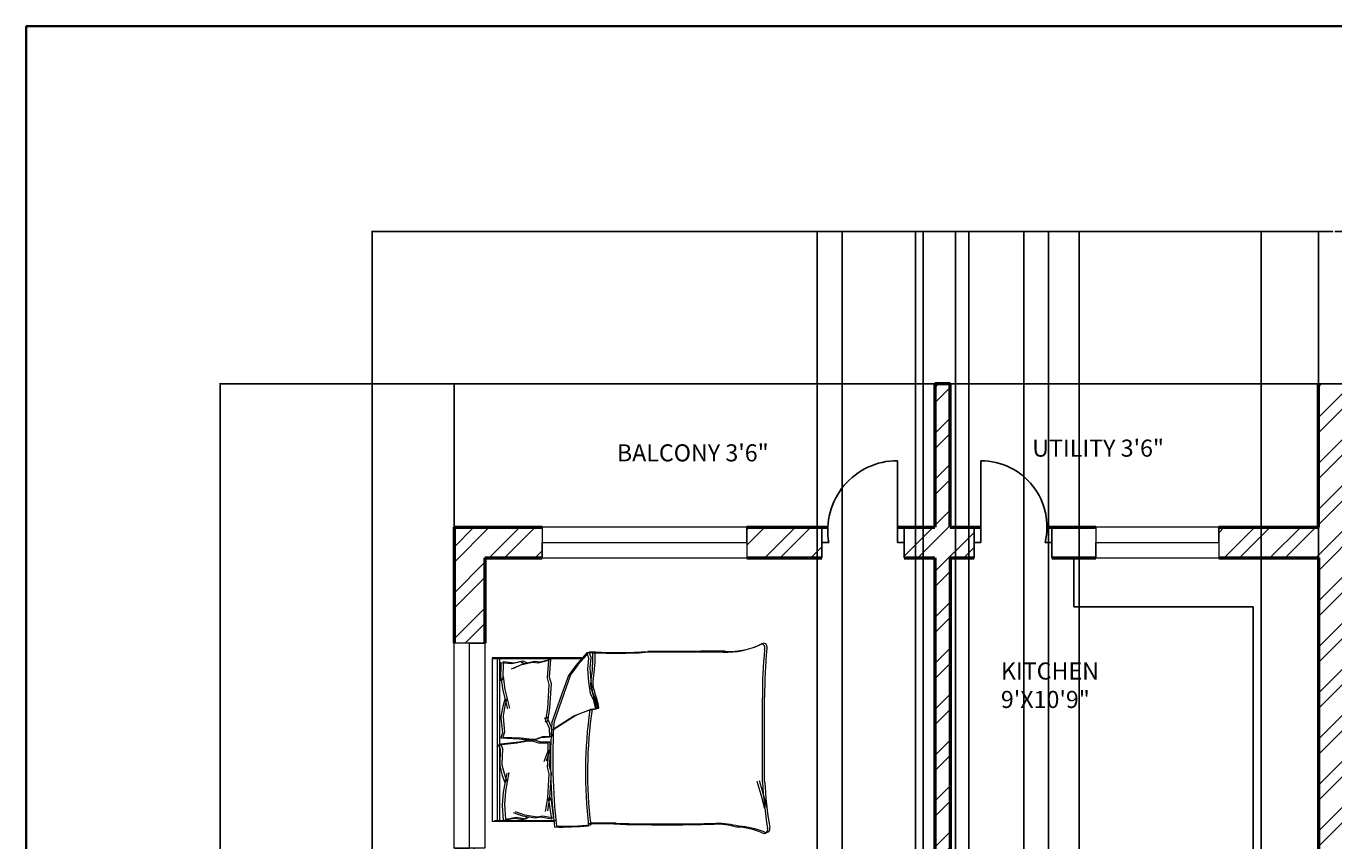
# Model space of a CAD drawing. Units: inches. Extents: x 1980 to 2738, y 1471 to 2568.
# Tile 19 of 22: x 1980 to 2363, y 2329 to 2568. Entities that reach past the tile are written whole.
import ezdxf

# ---------------------------------------------------------------- set-up
doc = ezdxf.new("R2010")
doc.units = ezdxf.units.IN
for name, color, linetype, lineweight in [('A-ANNO-DIMS', 2, 'Continuous', 18), ('A-ANNO-TTLB', 7, 'Continuous', 35), ('A-AREA-IDEN', 7, 'Continuous', 18), ('A-DOOR', 31, 'Continuous', 25), ('A-FLOR-BALC', 7, 'Continuous', 25), ('A-FLOR-CASE', 8, 'Continuous', 25), ('A-FURN', 8, 'Continuous', 18), ('A-GLAZ', 141, 'Continuous', 18), ('A-WALL', 7, 'Continuous', 50)]:
    doc.layers.add(name, color=color, linetype=linetype, lineweight=lineweight)
doc.layers.add('A-WALL-PATT', color=9, linetype='Continuous', lineweight=13, true_color=0xd19cc7)
doc.styles.get("Standard").update_dxf_attribs({"font": 'arial.ttf'})
doc.dimstyles.get("Standard").update_dxf_attribs({"dimtxt": 0.18, "dimasz": 0.18, "dimexe": 0.18, "dimexo": 0.0625, "dimgap": 0.09, "dimtad": 0, "dimtih": 1, "dimtoh": 1, "dimdec": 4, "dimzin": 0, "dimdsep": 46, "dimtxsty": 'Standard', "dimcen": 0.09, "dimadec": 0, "dimazin": 0, "dimtfac": 1, "dimtdec": 4, "dimtofl": 0, "dimtmove": 0, "dimatfit": 3, "dimfxl": 1, "dimtolj": 1, "dimtzin": 0, "dimarcsym": 0})

# ---------------------------------------------------------------- blocks, each defined once
blk = doc.blocks.new('BED-DOUBLE')
for p, q in [((0, 51.49), (0.64, 51.49)), ((0, 51.27), (26.61, 51.27)), ((0, 51.27), (26.61, 51.27)), ((0, 51.27), (0, 3.48)), ((0.64, 51.49), (27.25, 51.49)), ((0.64, 51.49), (27.25, 51.49)), ((1.53, 3.48), (1.53, 51.27)), ((1.53, 3.48), (1.53, 51.27)), ((2.17, 3.7), (2.17, 51.49)), ((2.17, 3.7), (2.17, 51.49)), ((2.56, 50.11), (2.46, 44.71)), ((2.56, 50.11), (2.46, 44.71)), ((2.56, 50.11), (5.77, 49.73)), ((2.56, 50.11), (5.77, 49.73)), ((3.2, 50.34), (3.1, 44.94)), ((3.2, 50.34), (3.1, 44.94)), ((3.2, 50.34), (6.41, 49.96)), ((3.2, 50.34), (6.41, 49.96)), ((5.77, 49.73), (8.34, 50.33)), ((5.77, 49.73), (8.34, 50.33)), ((6.41, 49.96), (8.98, 50.56)), ((6.41, 49.96), (8.98, 50.56)), ((11.83, 50.11), (8.26, 49.31)), ((11.83, 50.11), (8.26, 49.31)), ((8.34, 50.33), (9.38, 49.81)), ((8.34, 50.33), (9.38, 49.81)), ((12.47, 50.34), (8.9, 49.54)), ((12.47, 50.34), (8.9, 49.54)), ((8.98, 50.56), (10.02, 50.04)), ((8.98, 50.56), (10.02, 50.04)), ((13.43, 49.92), (11.83, 50.11)), ((13.43, 49.92), (11.83, 50.11)), ((14.07, 50.15), (12.47, 50.34)), ((14.07, 50.15), (12.47, 50.34)), ((16.57, 50.7), (13.43, 49.92)), ((16.57, 50.7), (13.43, 49.92)), ((17.21, 50.93), (14.07, 50.15)), ((17.21, 50.93), (14.07, 50.15)), ((16.17, 45.57), (16.57, 50.7)), ((16.17, 45.57), (16.57, 50.7)), ((16.81, 45.8), (17.21, 50.93)), ((16.81, 45.79), (17.21, 50.93)), ((27.75, 52.87), (24.5, 49.16)), ((27.75, 52.87), (24.5, 49.16)), ((28.38, 53.1), (25.13, 49.39)), ((28.38, 53.1), (25.13, 49.39)), ((29.49, 52.95), (27.75, 52.87, 3.87)), ((29.49, 52.95), (27.75, 52.87, 3.87)), ((28.36, 51.33), (27.75, 52.87)), ((28.36, 51.33), (27.75, 52.87)), ((28.06, 48.23), (28.36, 51.33)), ((28.06, 48.23), (28.36, 51.33)), ((30.13, 53.18), (28.38, 53.1, 3.87)), ((30.13, 53.18), (28.38, 53.1, 3.87)), ((29, 51.56), (28.38, 53.1)), ((29, 51.56), (28.38, 53.1)), ((28.69, 48.46), (29, 51.56)), ((28.69, 48.46), (29, 51.56)), ((8.26, 49.31), (5.58, 48.13)), ((8.26, 49.31), (5.58, 48.13)), ((8.9, 49.54), (6.22, 48.36)), ((8.9, 49.54), (6.22, 48.36)), ((22.33, 46.22), (20.32, 40.64)), ((22.33, 46.22), (20.32, 40.64)), ((22.97, 46.45), (20.96, 40.87)), ((22.97, 46.45), (20.96, 40.87)), ((24.5, 49.16), (22.33, 46.22)), ((24.5, 49.16), (22.33, 46.22)), ((25.13, 49.39), (22.97, 46.45)), ((25.13, 49.39), (22.97, 46.45)), ((28.36, 44.36), (28.06, 48.23)), ((28.36, 44.36), (28.06, 48.23)), ((29, 44.59), (28.69, 48.46)), ((29, 44.59), (28.69, 48.46)), ((2.46, 44.71), (2.54, 45.71)), ((2.46, 44.71), (2.54, 45.71)), ((2.54, 45.71), (3.07, 41.91)), ((2.54, 45.71), (3.07, 41.91)), ((3.1, 44.94), (3.18, 45.94)), ((3.1, 44.94), (3.18, 45.94)), ((3.18, 45.94), (3.71, 42.14)), ((3.18, 45.94), (3.71, 42.14)), ((16.73, 43.61), (16.17, 45.57)), ((16.73, 43.61), (16.17, 45.57)), ((16.29, 36.6), (16.73, 43.61)), ((16.29, 36.6), (16.73, 43.61)), ((17.37, 43.83), (16.81, 45.8)), ((17.37, 43.83), (16.81, 45.79)), ((16.93, 36.82), (17.37, 43.83)), ((16.93, 36.82), (17.37, 43.83)), ((28.83, 40.95), (28.36, 44.36)), ((28.83, 40.95), (28.36, 44.36)), ((29.47, 41.18), (29, 44.59)), ((29.47, 41.18), (29, 44.59)), ((3.07, 41.91), (4.42, 36.5)), ((3.07, 41.91), (4.42, 36.5)), ((3.67, 39.2), (3.08, 37.14)), ((3.67, 39.2), (3.08, 37.14)), ((3.71, 42.14), (5.06, 36.72)), ((3.71, 42.14), (5.06, 36.72)), ((4.31, 39.43), (3.72, 37.36)), ((4.31, 39.43), (3.72, 37.36)), ((20.32, 40.64), (17.38, 32.31)), ((20.32, 40.64), (17.38, 32.31)), ((20.96, 40.87), (18.02, 32.53)), ((20.96, 40.87), (18.02, 32.53)), ((29.76, 38.94), (28.83, 40.95)), ((29.76, 38.94), (28.83, 40.95)), ((30.4, 39.17), (29.47, 41.18)), ((30.4, 39.17), (29.47, 41.18)), ((30.38, 36.46), (29.76, 38.94)), ((30.38, 36.46), (29.76, 38.94)), ((31.02, 36.69), (30.4, 39.17)), ((31.02, 36.69), (30.4, 39.17)), ((79.24, 15.06), (79.24, 39.68)), ((79.24, 15.06), (79.24, 39.68)), ((79.88, 15.29), (79.88, 39.91)), ((79.88, 15.29), (79.88, 39.91)), ((3.08, 37.14), (2.54, 34.2)), ((3.08, 37.14), (2.54, 34.2)), ((3.72, 37.36), (3.18, 34.43)), ((3.72, 37.36), (3.18, 34.43)), ((15.63, 32.56), (16.29, 36.6)), ((15.63, 32.56), (16.29, 36.6)), ((16.27, 32.79), (16.93, 36.82)), ((16.27, 32.79), (16.93, 36.82)), ((18.02, 30.49), (24.52, 34.68)), ((18.02, 30.49), (24.52, 34.68)), ((23.88, 34.45), (28.36, 36.15)), ((23.88, 34.45), (28.36, 36.15)), ((24.52, 34.68), (29, 36.38)), ((24.52, 34.68), (29, 36.38)), ((28.36, 36.15), (30.38, 36.46)), ((28.36, 36.15), (30.38, 36.46)), ((29, 36.38), (31.02, 36.69)), ((29, 36.38), (31.02, 36.69)), ((2.54, 34.2), (2.56, 33.88)), ((2.54, 34.2), (2.56, 33.88)), ((2.56, 33.88), (2.98, 29.46)), ((2.56, 33.88), (2.98, 29.46)), ((3.18, 34.43), (3.2, 34.11)), ((3.18, 34.43), (3.2, 34.11)), ((3.2, 34.11), (3.62, 29.68)), ((3.2, 34.11), (3.62, 29.68)), ((16.74, 30.75), (15.45, 33.82)), ((16.74, 30.75), (15.45, 33.82)), ((17.38, 30.98), (16.09, 34.05)), ((17.38, 30.98), (16.09, 34.05)), ((16.89, 28.3), (16.74, 30.75)), ((16.89, 28.3), (16.74, 30.75)), ((17.38, 30.26), (23.88, 34.45)), ((17.38, 30.26), (23.88, 34.45)), ((17.53, 28.53), (17.38, 30.98)), ((17.53, 28.53), (17.38, 30.98)), ((2.98, 29.46), (2.49, 27.98)), ((2.98, 29.46), (2.49, 27.98)), ((2.49, 27.98), (7.87, 27.73)), ((2.49, 27.98), (7.87, 27.73)), ((3.62, 29.68), (3.13, 28.21)), ((3.62, 29.68), (3.13, 28.21)), ((3.13, 28.21), (8.51, 27.96)), ((3.13, 28.21), (8.51, 27.96)), ((7.22, 26.56), (10.4, 27.14)), ((7.22, 26.56), (10.4, 27.14)), ((7.86, 26.79), (11.04, 27.37)), ((7.86, 26.79), (11.04, 27.37)), ((7.87, 27.73), (11.08, 27.36)), ((7.87, 27.73), (11.08, 27.35)), ((8.51, 27.96), (11.72, 27.58)), ((8.51, 27.96), (11.72, 27.58)), ((10.4, 27.14), (11.7, 27.14)), ((10.4, 27.14), (11.7, 27.14)), ((11.04, 27.37), (12.34, 27.37)), ((11.04, 27.37), (12.34, 27.37)), ((11.08, 27.36), (12.38, 27.44)), ((11.08, 27.35), (12.38, 27.44)), ((11.7, 27.14), (13.58, 26.56)), ((11.7, 27.14), (13.58, 26.56)), ((11.72, 27.58), (13.02, 27.66)), ((11.72, 27.58), (13.02, 27.66)), ((12.34, 27.37), (14.22, 26.79)), ((12.34, 27.37), (14.22, 26.79)), ((12.38, 27.44), (14.22, 28.13)), ((12.38, 27.44), (14.22, 28.13)), ((13.02, 27.66), (14.86, 28.36)), ((13.02, 27.66), (14.86, 28.36)), ((14.22, 28.13), (16.89, 28.3)), ((14.22, 28.13), (16.89, 28.3)), ((14.86, 28.36), (17.53, 28.53)), ((14.86, 28.36), (17.53, 28.53)), ((1.87, 25.98), (7.22, 26.56)), ((1.87, 25.98), (7.22, 26.56)), ((2.45, 24.54), (1.87, 25.98)), ((2.45, 24.54), (1.87, 25.98)), ((2.3, 20.09), (2.45, 24.54)), ((2.3, 20.09), (2.45, 24.54)), ((2.51, 26.21), (7.86, 26.79)), ((2.51, 26.21), (7.86, 26.79)), ((3.09, 24.77), (2.51, 26.21)), ((3.09, 24.77), (2.51, 26.21)), ((2.94, 20.32), (3.09, 24.77)), ((2.94, 20.32), (3.09, 24.77)), ((13.58, 26.56), (16.26, 26.56)), ((13.58, 26.56), (16.26, 26.56)), ((14.22, 26.79), (16.9, 26.79)), ((14.22, 26.79), (16.9, 26.79)), ((16.26, 24.1), (15.17, 20.96)), ((16.26, 24.1), (15.17, 20.96)), ((16.9, 24.33), (15.81, 21.19)), ((16.9, 24.33), (15.81, 21.19)), ((16.17, 19.38), (16.57, 24.52)), ((16.17, 19.38), (16.57, 24.52)), ((16.26, 26.56), (16.26, 24.1)), ((16.26, 26.56), (16.26, 24.1)), ((16.81, 19.61), (17.21, 24.74)), ((16.81, 19.61), (17.21, 24.74)), ((16.9, 26.79), (16.9, 24.33)), ((16.9, 26.79), (16.9, 24.33)), ((2.3, 19.77), (2.3, 20.09)), ((2.3, 19.77), (2.3, 20.09)), ((3.03, 16.88), (2.3, 19.77)), ((3.03, 16.88), (2.3, 19.77)), ((2.94, 20), (2.94, 20.32)), ((2.94, 20), (2.94, 20.32)), ((3.67, 17.11), (2.94, 20)), ((3.67, 17.11), (2.94, 20)), ((16.73, 17.42), (16.17, 19.38)), ((16.73, 17.42), (16.17, 19.38)), ((17.37, 17.65), (16.81, 19.61)), ((17.37, 17.65), (16.81, 19.61)), ((3.75, 14.86), (3.03, 16.88)), ((3.75, 14.85), (3.03, 16.88)), ((3.32, 12.11), (4.33, 17.6)), ((3.32, 12.11), (4.33, 17.6)), ((4.39, 15.08), (3.67, 17.11)), ((4.39, 15.08), (3.67, 17.11)), ((3.96, 12.34), (4.97, 17.83)), ((3.96, 12.34), (4.97, 17.83)), ((16.29, 10.41), (16.73, 17.42)), ((16.29, 10.41), (16.73, 17.42)), ((16.93, 10.64), (17.37, 17.65)), ((16.93, 10.64), (17.37, 17.65)), ((3.03, 8.29), (3.32, 12.11)), ((3.03, 8.28), (3.32, 12.11)), ((3.67, 8.51), (3.96, 12.34)), ((3.67, 8.51), (3.96, 12.34)), ((3.01, 8.18), (3.03, 8.29)), ((3.01, 8.18), (3.03, 8.28)), ((3.34, 3.9), (3.01, 8.18)), ((3.34, 3.9), (3.01, 8.18)), ((3.65, 8.41), (3.67, 8.51)), ((3.65, 8.41), (3.67, 8.51)), ((3.98, 4.13), (3.65, 8.41)), ((3.98, 4.13), (3.65, 8.41)), ((15.63, 6.38), (16.29, 10.41)), ((15.63, 6.38), (16.29, 10.41)), ((16.27, 6.61), (16.93, 10.64)), ((16.27, 6.61), (16.93, 10.64)), ((16.29, 10.41), (16.62, 9.28)), ((16.29, 10.41), (16.62, 9.28)), ((16.62, 9.28), (17.34, 4.18)), ((16.62, 9.28), (17.34, 4.18)), ((16.93, 10.64), (17.26, 9.51)), ((16.93, 10.64), (17.26, 9.51)), ((17.26, 9.51), (17.98, 4.41)), ((17.26, 9.51), (17.98, 4.41)), ((3.32, 3.89), (6.5, 4.47)), ((3.32, 3.89), (6.5, 4.47)), ((3.96, 4.12), (7.14, 4.7)), ((3.96, 4.12), (7.14, 4.7)), ((8.95, 5.05), (6.21, 6.06)), ((8.95, 5.05), (6.21, 6.06)), ((6.5, 4.47), (9.1, 4.04)), ((6.5, 4.47), (9.1, 4.04)), ((9.59, 5.28), (6.85, 6.29)), ((9.59, 5.28), (6.85, 6.29)), ((7.14, 4.7), (9.74, 4.27)), ((7.14, 4.7), (9.74, 4.27)), ((12.57, 4.47), (8.95, 5.05)), ((12.57, 4.47), (8.95, 5.05)), ((9.1, 4.04), (10.11, 4.62)), ((9.1, 4.04), (10.11, 4.62)), ((13.21, 4.7), (9.59, 5.28)), ((13.21, 4.7), (9.59, 5.28)), ((9.74, 4.27), (10.75, 4.85)), ((9.74, 4.27), (10.75, 4.85)), ((14.16, 4.76), (12.57, 4.47)), ((14.16, 4.76), (12.57, 4.47)), ((14.8, 4.99), (13.21, 4.7)), ((14.8, 4.99), (13.21, 4.7)), ((17.34, 4.18), (14.16, 4.76)), ((17.34, 4.18), (14.16, 4.76)), ((17.98, 4.41), (14.8, 4.99)), ((17.98, 4.41), (14.8, 4.99)), ((18.11, 3.48), (0, 3.48)), ((18.11, 3.48), (0, 3.48)), ((18.75, 3.7), (0.64, 3.7)), ((18.75, 3.7), (0.64, 3.7))]:
    blk.add_line(p, q)
for centre, radius, start, end in [((68.67, 76.16), 23.07, 267.4714, 296.4681), ((68.67, 76.16), 23.07, 267.4714, 296.4681), ((69.31, 76.39), 23.07, 267.4714, 296.4681), ((69.31, 76.39), 23.07, 267.4714, 296.4681), ((78.87, 54.41), 1.1, 332.6588, 86.02), ((78.87, 54.41), 1.1, 332.6588, 86.02), ((212.28, 41.15), 133.04, 174.4998, 180.6351), ((212.28, 41.15), 133.04, 174.4998, 180.6351), ((79.51, 54.64), 1.1, 332.6588, 86.02), ((79.51, 54.64), 1.1, 332.6588, 86.02), ((212.92, 41.38), 133.04, 174.4998, 180.6351), ((212.92, 41.38), 133.04, 174.4998, 180.6351), ((-6.66, 51.33), 36.18, 349.8763, 2.5657), ((-6.66, 51.33), 36.18, 349.8763, 2.5657), ((36.31, 182.27), 129.5, 266.9791, 273.8365), ((36.31, 182.27), 129.5, 266.9791, 273.8365), ((-6.02, 51.56), 36.18, 349.8763, 2.5657), ((-6.02, 51.56), 36.18, 349.8763, 2.5657), ((36.95, 182.49), 129.5, 266.9791, 273.8365), ((36.95, 182.49), 129.5, 266.9791, 273.8365), ((67.82, -4508.74), 4561.86, 90.00217, 90.28689), ((67.82, -4508.74), 4561.86, 90.00217, 90.28689), ((68.46, -4508.51), 4561.86, 90.00217, 90.28689), ((68.46, -4508.52), 4561.86, 90.00217, 90.28689), ((35.07, 43.74), 6.22, 168.6608, 203.7384), ((35.07, 43.74), 6.22, 168.6608, 203.7384), ((35.71, 43.97), 6.22, 168.6608, 203.7384), ((35.71, 43.97), 6.22, 168.6608, 203.7384), ((1.48, 31.15), 29.65, 10.6617, 19.8806), ((1.48, 31.15), 29.65, 10.6617, 19.8806), ((2.12, 31.38), 29.65, 10.6617, 19.8806), ((2.12, 31.38), 29.65, 10.6617, 19.8806), ((156.32, 17.76), 129.02, 171.7845, 186.9006), ((156.32, 17.76), 129.02, 171.7845, 186.9006), ((156.96, 17.98), 129.02, 171.7845, 186.9006), ((156.96, 17.98), 129.02, 171.7845, 186.9006), ((30.44, 36.64), 0.185, 250.2464, 1.1377), ((30.44, 36.64), 0.185, 250.2464, 1.1377), ((31.08, 36.86), 0.185, 250.2464, 1.1377), ((31.08, 36.86), 0.185, 250.2464, 1.1377), ((182.05, 21.36), 164.97, 176.0865, 186.7821), ((182.05, 21.36), 164.97, 176.0865, 186.7821), ((182.69, 21.59), 164.97, 176.0865, 186.7821), ((182.69, 21.59), 164.97, 176.0865, 186.7821), ((-23.07, -16.99), 106.46, 13.3832, 17.7053), ((-23.07, -16.99), 106.46, 13.3832, 17.7053), ((-23.71, -17.22), 106.46, 13.3832, 17.7053), ((-23.71, -17.22), 106.46, 13.3832, 17.7053), ((200.84, 21.43), 121.76, 182.9958, 189.4091), ((200.84, 21.43), 121.76, 182.9958, 189.4091), ((201.48, 21.66), 121.76, 182.9958, 189.4091), ((201.48, 21.66), 121.76, 182.9958, 189.4091), ((20.1, 85.16), 83.31, 268.7218, 275.604), ((20.1, 85.16), 83.31, 268.7218, 275.604), ((20.74, 85.39), 83.31, 268.7218, 275.604), ((20.74, 85.39), 83.31, 268.7218, 275.604), ((31.17, -167.31), 170.11, 88.4762, 91.0082), ((31.17, -167.31), 170.11, 88.4762, 91.0082), ((31.81, -167.08), 170.11, 88.4762, 91.0082), ((31.81, -167.08), 170.11, 88.4762, 91.0082), ((50.61, 484.82), 482.31, 268.2277, 271.7185), ((50.61, 484.82), 482.31, 268.2277, 271.7185), ((51.25, 485.05), 482.31, 268.2277, 271.7185), ((51.25, 485.05), 482.31, 268.2277, 271.7185), ((64.51, -26.9), 29.63, 76.0648, 88.9113), ((64.51, -26.9), 29.63, 76.0648, 88.9113), ((65.15, -26.67), 29.63, 76.0648, 88.9113), ((65.15, -26.67), 29.63, 76.0648, 88.9113), ((70.28, -21.66), 23.56, 67.9751, 86.652), ((70.28, -21.66), 23.56, 67.9751, 86.652), ((70.91, -21.43), 23.56, 67.9751, 86.652), ((70.91, -21.43), 23.56, 67.9751, 86.652), ((79.72, 1.09), 1.09, 236.1736, 23.4781), ((79.72, 1.09), 1.09, 236.1736, 23.4781), ((80.36, 1.32), 1.09, 236.1736, 23.4781), ((80.36, 1.32), 1.09, 236.1736, 23.4781)]:
    blk.add_arc(centre, radius, start, end)
blk = doc.blocks.new('WIN-60IN-WALL')
for p, q in [((0, 9), (0, 0)), ((60, 9), (0, 9)), ((60, 4.5), (60, 9)), ((60, 9), (60, 0)), ((0, 0), (0, 4.5)), ((0, 4.5), (60, 4.5)), ((0, 0), (60, 0))]:
    blk.add_line(p, q)
blk = doc.blocks.new('*D35')
at = {"layer": 'A-ANNO-DIMS', "color": 0, "lineweight": -2, "transparency": 16777216}
for p, q in [((2081.08, 2291.77), (2081.08, 2507.54)), ((2081.26, 2507.36), (2362.79, 2507.36)), ((2644.9, 2507.36), (2363.37, 2507.36)), ((2645.08, 2291.77), (2645.08, 2507.54))]:
    blk.add_line(p, q, dxfattribs=at)
at = {"layer": 'A-ANNO-DIMS', "color": 0, "transparency": 16777216}
for points in [[(2081.26, 2507.39), (2081.26, 2507.33), (2081.08, 2507.36)], [(2644.9, 2507.39), (2644.9, 2507.33), (2645.08, 2507.36)]]:
    blk.add_solid(points, dxfattribs=at)
at = {"layer": 'Defpoints', "color": 0, "transparency": 16777216}
for p in [(2645.08, 2507.36), (2081.08, 2291.71), (2645.08, 2291.71)]:
    blk.add_point(p, dxfattribs=at)
at = {"layer": 'A-ANNO-DIMS', "color": 0, "transparency": 16777216, "insert": (2363.08, 2507.36), "char_height": 0.18, "attachment_point": 5}
blk.add_mtext('\\A1;564', dxfattribs=at)
blk = doc.blocks.new('*D36')
at = {"layer": 'A-ANNO-DIMS', "color": 0, "lineweight": -2, "transparency": 16777216}
for p, q in [((2105.02, 2462.71), (2036.25, 2462.71)), ((2036.43, 2462.53), (2036.43, 2053.39)), ((2036.43, 1643.89), (2036.43, 2053.02)), ((2105.02, 1643.71), (2036.25, 1643.71))]:
    blk.add_line(p, q, dxfattribs=at)
at = {"layer": 'A-ANNO-DIMS', "color": 0, "transparency": 16777216}
for points in [[(2036.4, 2462.53), (2036.46, 2462.53), (2036.43, 2462.71)], [(2036.4, 1643.89), (2036.46, 1643.89), (2036.43, 1643.71)]]:
    blk.add_solid(points, dxfattribs=at)
at = {"layer": 'Defpoints', "color": 0, "transparency": 16777216}
for p in [(2036.43, 2462.71), (2105.08, 2462.71), (2105.08, 1643.71)]:
    blk.add_point(p, dxfattribs=at)
at = {"layer": 'A-ANNO-DIMS', "color": 0, "transparency": 16777216, "insert": (2036.43, 2053.21), "char_height": 0.18, "attachment_point": 5}
blk.add_mtext('\\A1;819', dxfattribs=at)
blk = doc.blocks.new('*D44')
at = {"layer": 'A-ANNO-DIMS', "color": 0, "lineweight": -2, "transparency": 16777216}
for p, q in [((2218.88, 1694.77), (2218.88, 2507.54)), ((2219.06, 2507.36), (2229.18, 2507.36)), ((2240.22, 2507.36), (2230.11, 2507.36)), ((2240.4, 1694.77), (2240.4, 2507.54))]:
    blk.add_line(p, q, dxfattribs=at)
at = {"layer": 'A-ANNO-DIMS', "color": 0, "transparency": 16777216}
for points in [[(2219.06, 2507.39), (2219.06, 2507.33), (2218.88, 2507.36)], [(2240.22, 2507.39), (2240.22, 2507.33), (2240.4, 2507.36)]]:
    blk.add_solid(points, dxfattribs=at)
at = {"layer": 'Defpoints', "color": 0, "transparency": 16777216}
for p in [(2240.4, 2507.36), (2218.88, 1694.71), (2240.4, 1694.71)]:
    blk.add_point(p, dxfattribs=at)
at = {"layer": 'A-ANNO-DIMS', "color": 0, "transparency": 16777216, "insert": (2229.64, 2507.36), "char_height": 0.18, "attachment_point": 5}
blk.add_mtext('\\A1;21.525', dxfattribs=at)
blk = doc.blocks.new('*D45')
at = {"layer": 'A-ANNO-DIMS', "color": 0, "lineweight": -2, "transparency": 16777216}
for p, q in [((2255.99, 1694.77), (2255.99, 2507.54)), ((2256.17, 2507.36), (2267.22, 2507.36)), ((2279.21, 2507.36), (2268.15, 2507.36)), ((2279.39, 1694.77), (2279.39, 2507.54))]:
    blk.add_line(p, q, dxfattribs=at)
at = {"layer": 'A-ANNO-DIMS', "color": 0, "transparency": 16777216}
for points in [[(2256.17, 2507.39), (2256.17, 2507.33), (2255.99, 2507.36)], [(2279.21, 2507.39), (2279.21, 2507.33), (2279.39, 2507.36)]]:
    blk.add_solid(points, dxfattribs=at)
at = {"layer": 'Defpoints', "color": 0, "transparency": 16777216}
for p in [(2279.39, 2507.36), (2255.99, 1694.71), (2279.39, 1694.71)]:
    blk.add_point(p, dxfattribs=at)
at = {"layer": 'A-ANNO-DIMS', "color": 0, "transparency": 16777216, "insert": (2267.69, 2507.36), "char_height": 0.18, "attachment_point": 5}
blk.add_mtext('\\A1;23.407', dxfattribs=at)
blk = doc.blocks.new('*D46')
at = {"layer": 'A-ANNO-DIMS', "color": 0, "lineweight": -2, "transparency": 16777216}
for p, q in [((2211.52, 1814.77), (2211.52, 2507.54)), ((2211.7, 2507.36), (2226.69, 2507.36)), ((2242.46, 2507.36), (2227.48, 2507.36)), ((2242.64, 1814.77), (2242.64, 2507.54))]:
    blk.add_line(p, q, dxfattribs=at)
at = {"layer": 'A-ANNO-DIMS', "color": 0, "transparency": 16777216}
for points in [[(2211.7, 2507.39), (2211.7, 2507.33), (2211.52, 2507.36)], [(2242.46, 2507.39), (2242.46, 2507.33), (2242.64, 2507.36)]]:
    blk.add_solid(points, dxfattribs=at)
at = {"layer": 'Defpoints', "color": 0, "transparency": 16777216}
for p in [(2242.64, 2507.36), (2211.52, 1814.71), (2242.64, 1814.71)]:
    blk.add_point(p, dxfattribs=at)
at = {"layer": 'A-ANNO-DIMS', "color": 0, "transparency": 16777216, "insert": (2227.08, 2507.36), "char_height": 0.18, "attachment_point": 5}
blk.add_mtext('\\A1;31.12', dxfattribs=at)
blk = doc.blocks.new('*D50')
at = {"layer": 'A-ANNO-DIMS', "color": 0, "lineweight": -2, "transparency": 16777216}
for p, q in [((2288.43, 1708.09), (2288.43, 2507.54)), ((2288.61, 2507.36), (2314.71, 2507.36)), ((2341.6, 2507.36), (2315.5, 2507.36)), ((2341.78, 1708.09), (2341.78, 2507.54))]:
    blk.add_line(p, q, dxfattribs=at)
at = {"layer": 'A-ANNO-DIMS', "color": 0, "transparency": 16777216}
for points in [[(2288.61, 2507.39), (2288.61, 2507.33), (2288.43, 2507.36)], [(2341.6, 2507.39), (2341.6, 2507.33), (2341.78, 2507.36)]]:
    blk.add_solid(points, dxfattribs=at)
at = {"layer": 'Defpoints', "color": 0, "transparency": 16777216}
for p in [(2341.78, 2507.36), (2288.43, 1708.03), (2341.78, 1708.03)]:
    blk.add_point(p, dxfattribs=at)
at = {"layer": 'A-ANNO-DIMS', "color": 0, "transparency": 16777216, "insert": (2315.11, 2507.36), "char_height": 0.18, "attachment_point": 5}
blk.add_mtext('\\A1;53.34', dxfattribs=at)
blk = doc.blocks.new('*D51')
at = {"layer": 'A-ANNO-DIMS', "color": 0, "lineweight": -2, "transparency": 16777216}
for p, q in [((2341.78, 1708.09), (2341.78, 2507.54)), ((2341.96, 2507.36), (2349.72, 2507.36)), ((2358.4, 2507.36), (2350.63, 2507.36)), ((2358.58, 1694.77), (2358.58, 2507.54))]:
    blk.add_line(p, q, dxfattribs=at)
at = {"layer": 'A-ANNO-DIMS', "color": 0, "transparency": 16777216}
for points in [[(2341.96, 2507.39), (2341.96, 2507.33), (2341.78, 2507.36)], [(2358.4, 2507.39), (2358.4, 2507.33), (2358.58, 2507.36)]]:
    blk.add_solid(points, dxfattribs=at)
at = {"layer": 'Defpoints', "color": 0, "transparency": 16777216}
for p in [(2358.58, 2507.36), (2341.78, 1708.03), (2358.58, 1694.71)]:
    blk.add_point(p, dxfattribs=at)
at = {"layer": 'A-ANNO-DIMS', "color": 0, "transparency": 16777216, "insert": (2350.18, 2507.36), "char_height": 0.18, "attachment_point": 5}
blk.add_mtext('\\A1;16.807', dxfattribs=at)
blk = doc.blocks.new('*D54')
at = {"layer": 'A-ANNO-DIMS', "color": 0, "lineweight": -2, "transparency": 16777216}
for p, q in [((2252.1, 1949.01), (2252.1, 2507.54)), ((2252.28, 2507.36), (2261.78, 2507.36)), ((2272.03, 2507.36), (2262.53, 2507.36)), ((2272.21, 1949.01), (2272.21, 2507.54))]:
    blk.add_line(p, q, dxfattribs=at)
at = {"layer": 'A-ANNO-DIMS', "color": 0, "transparency": 16777216}
for points in [[(2252.28, 2507.39), (2252.28, 2507.33), (2252.1, 2507.36)], [(2272.03, 2507.39), (2272.03, 2507.33), (2272.21, 2507.36)]]:
    blk.add_solid(points, dxfattribs=at)
at = {"layer": 'Defpoints', "color": 0, "transparency": 16777216}
for p in [(2272.21, 2507.36), (2252.1, 1948.95), (2272.21, 1948.95)]:
    blk.add_point(p, dxfattribs=at)
at = {"layer": 'A-ANNO-DIMS', "color": 0, "transparency": 16777216, "insert": (2262.16, 2507.36), "char_height": 0.18, "attachment_point": 5}
blk.add_mtext('\\A1;20.11', dxfattribs=at)

msp = doc.modelspace()

# ---------------------------------------------------------------- hatches: boundary and pattern name
at = {"layer": 'A-WALL-PATT'}
h = msp.add_hatch(dxfattribs=at)
h.set_pattern_fill('ANSI32', color=256)
h.paths.add_polyline_path([(2257.5661, 2416.2064), (2257.5661, 2420.7064), (2250.5833, 2420.7064), (2250.5833, 2462.7064), (2246.0833, 2462.7064), (2246.0833, 2420.7064), (2237.0791, 2420.7064), (2237.0791, 2411.7064), (2246.0833, 2411.7064), (2246.0833, 2291.7064), (2242.6109, 2291.7064), (2242.6109, 2287.2064), (2246.0833, 2287.2064), (2250.5833, 2287.2064), (2250.5833, 2291.7064), (2250.5833, 2411.7064), (2257.5661, 2411.7064)])
h.paths.add_polyline_path([(2387.0396, 2416.2064), (2387.0396, 2420.7064), (2367.5833, 2420.7064), (2367.5833, 2462.7064), (2358.5833, 2462.7064), (2358.5833, 2420.7064), (2329.3087, 2420.7064), (2329.3087, 2411.7064), (2358.5833, 2411.7064), (2358.5833, 2321.7275), (2358.5833, 2309.7064), (2347.3089, 2309.7064), (2293.3089, 2309.7064), (2293.3089, 2259.0771), (2297.8089, 2259.0771), (2297.8089, 2305.2064), (2347.3089, 2305.2064), (2347.3089, 2284.7412), (2351.8089, 2284.7412), (2351.8089, 2305.2064), (2372.3188, 2305.2064), (2372.3761, 2284.3899), (2377.0295, 2284.3899), (2377.0295, 2299.3058), (2377.0295, 2305.2064), (2426.5295, 2305.2064), (2426.5295, 2257.5573), (2431.0295, 2257.5573), (2431.0295, 2309.7064), (2377.0295, 2309.7064), (2367.5833, 2309.7064), (2367.5833, 2321.7275), (2367.5833, 2411.7064), (2387.0396, 2411.7064)])
h.paths.add_polyline_path([(2448.5267, 2416.2064), (2448.5267, 2420.7064), (2423.0396, 2420.7064), (2423.0396, 2411.7064), (2448.5267, 2411.7064)])
h.paths.add_polyline_path([(2130.9128, 2416.2064), (2130.9128, 2420.7064), (2105.0833, 2420.7064), (2105.0833, 2386.6942), (2114.0833, 2386.6942), (2114.0833, 2411.7064), (2130.9128, 2411.7064)])
h.paths.add_polyline_path([(2212.9478, 2420.7064), (2190.9128, 2420.7064), (2190.9128, 2411.7064), (2212.9478, 2411.7064), (2212.9478, 2416.2064)])
h.paths.add_polyline_path([(2114.0833, 2326.6942), (2105.0833, 2326.6942), (2105.0833, 2291.7064), (2081.0833, 2291.7064), (2081.0833, 2287.2064), (2105.0833, 2287.2064), (2105.0833, 2276.1935), (2114.0833, 2276.1935), (2114.0833, 2287.2064), (2166.3825, 2287.2064), (2166.3825, 2289.4564), (2166.3825, 2291.7064), (2114.0833, 2291.7064)])
h.paths.add_polyline_path([(2114.0833, 2252.1935), (2105.0833, 2252.1935), (2105.0833, 2233.2064), (2081.0833, 2233.2064), (2081.0833, 2228.7064), (2105.0833, 2228.7064), (2105.0833, 2213.4478), (2114.0833, 2213.4478), (2114.0833, 2228.7064), (2195.0833, 2228.7064), (2199.5833, 2228.7064), (2208.4455, 2228.7064), (2208.4455, 2230.9564), (2208.4455, 2233.2064), (2199.5833, 2233.2064), (2199.5833, 2287.2064), (2206.8904, 2287.2064), (2206.8904, 2289.4564), (2206.8904, 2291.7064), (2189.446, 2291.7064), (2189.446, 2289.4564), (2189.446, 2287.2064), (2195.0833, 2287.2064), (2195.0833, 2233.2064), (2114.0833, 2233.2064)])
h.paths.add_polyline_path([(2114.0833, 2153.4478), (2109.5833, 2153.4478), (2105.0833, 2153.4478), (2105.0833, 2135.2374), (2114.0833, 2135.2374)], flags=17)
h.paths.add_polyline_path([(2135.9619, 2095.4081), (2140.1805, 2095.4081), (2140.1805, 2104.2064), (2114.0833, 2104.2064), (2114.0833, 2110.3997), (2109.5833, 2110.3997), (2105.0833, 2110.3997), (2105.0833, 2104.2064), (2081.0833, 2104.2064), (2081.0833, 2099.7064), (2105.0833, 2099.7064), (2127.5416, 2099.8532), (2127.5416, 2056.9393), (2136.2133, 2056.9393)], flags=17)
h.paths.add_polyline_path([(2255.4895, 2104.2064), (2250.5833, 2104.2064), (2250.5833, 2233.2064), (2246.0833, 2233.2064), (2242.4941, 2233.2064), (2242.4941, 2228.7064), (2246.0833, 2228.7064), (2246.0833, 2104.2064), (2163.6825, 2104.2064), (2163.6825, 2099.8072), (2163.6825, 2095.4081), (2191.4325, 2095.4081), (2191.4325, 2011.2064), (2186.0833, 2011.2064), (2136.5143, 2010.8824), (2136.3702, 2032.9403), (2131.9559, 2032.9115), (2127.5416, 2032.8826), (2127.5416, 2006.7064), (2105.0833, 2006.7064), (2081.0833, 2006.7064), (2081.0833, 2002.2064), (2105.0833, 2002.2064), (2105.0833, 1995.9329), (2114.0833, 1995.9329), (2114.0833, 2002.2064), (2246.0833, 2002.2064), (2246.0833, 1877.7064), (2242.1358, 1877.7064), (2242.1358, 1873.2064), (2250.5833, 1873.2064), (2250.5833, 2002.2064), (2255.3335, 2002.2064), (2255.3335, 2011.2064), (2195.9325, 2011.2064), (2195.9325, 2095.2064), (2255.4895, 2095.2064), (2255.4895, 2099.5471)])
h.paths.add_polyline_path([(2199.5833, 1873.2064), (2209.827, 1873.2064), (2209.827, 1875.4564), (2209.827, 1877.7064), (2114.0833, 1877.7064), (2114.0833, 1890.0968), (2105.0833, 1890.0968), (2105.0833, 1877.7064), (2081.0833, 1877.7064), (2081.0833, 1873.2064), (2105.0833, 1873.2064), (2105.0833, 1857.7279), (2114.0833, 1857.7279), (2114.0833, 1873.2064), (2195.0833, 1873.2064), (2195.0833, 1819.2064), (2190.298, 1819.2064), (2190.298, 1814.7064), (2209.8976, 1814.7064), (2209.8976, 1816.9564), (2209.8976, 1819.2064), (2199.5833, 1819.2064)])
h.paths.add_polyline_path([(2114.0833, 1814.7064), (2166.2538, 1814.7064), (2166.2538, 1816.9564), (2166.2538, 1819.2064), (2114.0833, 1819.2064), (2114.0833, 1833.7279), (2109.5833, 1833.7279), (2105.0833, 1833.7279), (2105.0833, 1819.2064), (2081.0833, 1819.2064), (2081.0833, 1814.7064), (2105.0833, 1814.7064), (2105.0833, 1782.5516), (2114.0833, 1782.5516)])
h.paths.add_polyline_path([(2114.0833, 1722.5516), (2109.5833, 1722.5516), (2105.0833, 1722.5516), (2105.0833, 1685.7064), (2124.5104, 1685.7064), (2124.5104, 1690.2064), (2124.5104, 1694.7064), (2114.0833, 1694.7064)])
h.paths.add_polyline_path([(2218.8787, 1694.7064), (2184.5104, 1694.7064), (2184.5104, 1685.7064), (2218.8787, 1685.7064), (2218.8787, 1690.2064)])
h.paths.add_polyline_path([(2250.5833, 1819.2064), (2242.6431, 1819.2064), (2242.6431, 1816.9564), (2242.6431, 1814.7064), (2246.0833, 1814.7064), (2246.0833, 1694.7064), (2240.4035, 1694.7064), (2240.4035, 1690.2064), (2240.4035, 1685.7064), (2246.0833, 1685.7064), (2246.0833, 1643.7064), (2250.5833, 1643.7064), (2250.5833, 1685.7064), (2255.9859, 1685.7064), (2255.9859, 1690.2064), (2255.9859, 1694.7064), (2250.5833, 1694.7064)])
h.paths.add_polyline_path([(2297.4764, 1694.7064), (2279.3934, 1694.7064), (2279.3934, 1690.2064), (2279.3934, 1685.7064), (2297.4764, 1685.7064), (2297.4764, 1690.2064)])
h.paths.add_polyline_path([(2377.1596, 1694.7064), (2367.5833, 1694.7064), (2367.5833, 1787.7064), (2431.0295, 1787.7064), (2431.0295, 1792.2064), (2431.0295, 1849.4149), (2428.7795, 1849.4149), (2426.5295, 1849.4149), (2426.5295, 1792.2064), (2421.5833, 1792.2064), (2367.5833, 1792.2064), (2297.8089, 1792.2064), (2297.8089, 1850.2946), (2295.5589, 1850.2946), (2293.3089, 1850.2946), (2293.3089, 1792.2064), (2293.3089, 1787.7064), (2297.8089, 1787.7064), (2358.5833, 1787.7064), (2358.5833, 1694.7064), (2333.4764, 1694.7064), (2333.4764, 1685.7064), (2358.5833, 1685.7064), (2358.5833, 1643.7064), (2367.5833, 1643.7064), (2367.5833, 1685.7064), (2377.1596, 1685.7064)])
h.paths.add_polyline_path([(2442.4912, 1694.7064), (2413.1596, 1694.7064), (2413.1596, 1685.7064), (2442.4912, 1685.7064)])
h.paths.add_polyline_path([(2480.0833, 1814.7064), (2483.4816, 1814.7064), (2483.4816, 1817.9384), (2483.4816, 1819.2064), (2475.5833, 1819.2064), (2475.5833, 1694.7064), (2470.7283, 1694.7064), (2470.7283, 1685.7064), (2475.5833, 1685.7064), (2475.5833, 1643.7064), (2480.0833, 1643.7064), (2480.0833, 1685.7064), (2486.3293, 1685.7064), (2486.3293, 1690.2064), (2486.3293, 1694.7064), (2480.0833, 1694.7064)])
h.paths.add_polyline_path([(2621.0833, 1721.7349), (2612.0833, 1721.7349), (2612.0833, 1694.7064), (2586.1453, 1694.7064), (2586.1453, 1685.7064), (2621.0833, 1685.7064)])
h.paths.add_polyline_path([(2526.1453, 1690.2064), (2526.1453, 1694.7064), (2511.584, 1694.7064), (2511.584, 1690.2064), (2511.584, 1685.7064), (2526.1453, 1685.7064)])
h.paths.add_polyline_path([(2645.0833, 1819.2064), (2621.0833, 1819.2064), (2621.0833, 1835.8527), (2616.5833, 1835.8527), (2612.0833, 1835.8527), (2612.0833, 1819.2064), (2560.2541, 1819.2064), (2560.2541, 1814.7064), (2612.0833, 1814.7064), (2612.0833, 1781.7349), (2621.0833, 1781.7349), (2621.0833, 1814.7064), (2645.0833, 1814.7064)])
h.paths.add_polyline_path([(2645.0833, 1877.7064), (2621.0833, 1877.7064), (2621.0833, 1886.4375), (2612.0833, 1886.4375), (2612.0833, 1877.7064), (2517.1032, 1877.7064), (2517.1032, 1875.4564), (2517.1032, 1873.2064), (2526.5833, 1873.2064), (2526.5833, 1819.2064), (2516.6454, 1819.2064), (2516.6454, 1816.9564), (2516.6454, 1814.7064), (2536.4445, 1814.7064), (2536.4445, 1816.9564), (2536.4445, 1819.2064), (2531.0833, 1819.2064), (2531.0833, 1873.2064), (2612.0833, 1873.2064), (2612.0833, 1859.8527), (2621.0833, 1859.8527), (2621.0833, 1873.2064), (2645.0833, 1873.2064)])
h.paths.add_polyline_path([(2645.0833, 2006.7064), (2621.0833, 2006.7064), (2588.5085, 2006.7064), (2588.5085, 2052.9125), (2579.9045, 2052.9125), (2579.9045, 2011.2064), (2519.9045, 2011.2064), (2519.9045, 2095.2064), (2553.1204, 2095.2064), (2553.1204, 2104.2064), (2480.0833, 2104.2064), (2480.0833, 2228.7064), (2484.3832, 2228.7064), (2484.3832, 2230.9564), (2484.3832, 2233.2064), (2475.5833, 2233.2064), (2475.5833, 2104.2064), (2463.1308, 2104.2064), (2463.1308, 2095.2064), (2501.2463, 2095.2064), (2510.9045, 2095.2064), (2515.4045, 2095.2064), (2515.4045, 2011.2064), (2510.9045, 2011.2064), (2501.2463, 2011.2064), (2462.5957, 2011.2064), (2462.5957, 2002.2064), (2475.5833, 2002.2064), (2475.5833, 1873.2064), (2483.6146, 1873.2064), (2483.6146, 1875.4564), (2483.6146, 1877.7064), (2480.0833, 1877.7064), (2480.0833, 2002.2064), (2612.0833, 2002.2064), (2612.0833, 1996.309), (2621.0833, 1996.309), (2621.0833, 2002.2064), (2645.0833, 2002.2064)])
h.paths.add_polyline_path([(2588.5085, 2099.7277), (2621.0833, 2099.7277), (2645.0833, 2099.7064), (2645.0833, 2104.2064), (2621.0833, 2104.2064), (2621.0833, 2109.0038), (2616.5833, 2109.0038), (2612.0833, 2109.0038), (2612.0833, 2104.2064), (2575.0621, 2104.2064), (2575.0621, 2099.7064), (2575.0621, 2095.2064), (2579.9045, 2095.2064), (2579.9045, 2076.9125), (2588.5085, 2076.9125)], flags=17)
h.paths.add_polyline_path([(2367.5833, 2002.2064), (2373.7228, 2002.2064), (2373.7228, 2006.7064), (2373.7228, 2011.2064), (2350.7889, 2011.2064), (2350.7889, 2006.7064), (2350.7889, 2002.2064), (2358.5833, 2002.2064), (2358.5833, 1877.7064), (2293.3089, 1877.7064), (2293.3089, 1870.4987), (2297.8089, 1870.4987), (2297.8089, 1873.2064), (2347.3089, 1873.2064), (2347.3089, 1847.2208), (2351.8089, 1847.2208), (2351.8089, 1873.2064), (2372.5295, 1873.2064), (2372.5295, 1847.8619), (2377.0295, 1847.8619), (2377.0295, 1873.2064), (2426.5295, 1873.2064), (2426.5295, 1868.7339), (2431.0295, 1868.7339), (2431.0295, 1877.7064), (2367.5833, 1877.7064)])
h.paths.add_polyline_path([(2531.0833, 2287.2064), (2534.2285, 2287.2064), (2534.2285, 2291.7064), (2516.7886, 2291.7064), (2516.7886, 2287.2064), (2526.5833, 2287.2064), (2526.5833, 2233.2064), (2517.9112, 2233.2064), (2517.9112, 2230.9564), (2517.9112, 2228.7064), (2526.5833, 2228.7064), (2531.0833, 2228.7064), (2612.0833, 2228.7064), (2612.0833, 2206.8504), (2621.0833, 2206.8504), (2621.0833, 2228.7064), (2645.0833, 2228.7064), (2645.0833, 2233.2064), (2621.0833, 2233.2064), (2621.0833, 2241.8536), (2616.5833, 2241.8536), (2612.0833, 2241.8536), (2612.0833, 2233.2064), (2531.0833, 2233.2064)])
h.paths.add_polyline_path([(2645.0833, 2291.7064), (2621.0833, 2291.7064), (2621.0833, 2323.0138), (2616.5833, 2323.0138), (2612.0833, 2323.0138), (2612.0833, 2291.7064), (2559.6852, 2291.7064), (2559.6852, 2289.4564), (2559.6852, 2287.2064), (2612.0833, 2287.2064), (2612.0833, 2265.8536), (2621.0833, 2265.8536), (2621.0833, 2287.2064), (2645.0833, 2287.2064)])
h.paths.add_polyline_path([(2621.0833, 2420.7064), (2582.8189, 2420.7064), (2582.8189, 2411.7064), (2612.0833, 2411.7064), (2612.0833, 2383.0138), (2621.0833, 2383.0138)])
h.paths.add_polyline_path([(2480.0833, 2411.7064), (2485.7342, 2411.7064), (2485.7342, 2416.2064), (2485.7342, 2420.7064), (2480.0833, 2420.7064), (2480.0833, 2462.7064), (2475.5833, 2462.7064), (2475.5833, 2420.7064), (2469.4083, 2420.7064), (2469.4083, 2411.7064), (2475.5833, 2411.7064), (2475.5833, 2291.7064), (2475.5833, 2287.2064), (2482.9195, 2287.2064), (2482.9195, 2289.4564), (2482.9195, 2291.7064), (2480.0833, 2291.7064)])
h.paths.add_polyline_path([(2367.5833, 2228.7064), (2431.0295, 2228.7064), (2431.0295, 2233.2064), (2431.0295, 2237.4203), (2428.7795, 2237.4203), (2426.5295, 2237.4203), (2426.5295, 2233.2064), (2377.0295, 2233.2064), (2377.0295, 2260.3837), (2372.4423, 2260.3837), (2372.517, 2233.2635), (2351.8089, 2233.2064), (2351.8089, 2260.7412), (2347.3089, 2260.7412), (2347.3089, 2233.2064), (2297.8089, 2233.2064), (2297.8089, 2236.9324), (2293.3089, 2236.9324), (2293.3089, 2228.7064), (2358.5833, 2228.7064), (2358.5833, 2104.2064), (2353.3665, 2104.2064), (2353.3665, 2095.2064), (2373.8869, 2095.2064), (2373.8869, 2099.7064), (2373.8869, 2104.2064), (2367.5833, 2104.2064)])
h.paths.add_polyline_path([(2321.2323, 2104.2064), (2303.4895, 2104.2064), (2303.4895, 2095.2064), (2321.2323, 2095.2064), (2321.2323, 2099.7064)], flags=0)
h.paths.add_polyline_path([(2415.1308, 2099.7064), (2415.1308, 2104.2064), (2404.81, 2104.2064), (2404.81, 2095.2064), (2415.1308, 2095.2064)], flags=17)
h.paths.add_polyline_path([(2318.6336, 2011.2064), (2303.3335, 2011.2064), (2303.3335, 2002.2064), (2318.6336, 2002.2064)], flags=0)
h.paths.add_polyline_path([(2414.5957, 2011.2064), (2406.2461, 2011.2064), (2406.2461, 2006.7064), (2406.2461, 2002.2064), (2414.5957, 2002.2064)], flags=17)

# ---------------------------------------------------------------- linework, layer by layer
at = {"layer": 'A-ANNO-TTLB'}
msp.add_lwpolyline([(1979.5621, 2567.5568), (2738.2543, 2567.5568), (2738.2543, 1471.317), (1979.5621, 1471.317)], close=True, dxfattribs=at)
at = {"layer": 'A-DOOR'}
for p, q in [((2235.0791, 2416.2064), (2235.0791, 2440.2064)), ((2259.5661, 2416.2064), (2259.5661, 2440.2064)), ((2212.9478, 2420.7064), (2212.9478, 2411.7064)), ((2237.0791, 2420.7064), (2237.0791, 2411.7064)), ((2257.5661, 2420.7064), (2257.5661, 2411.7064)), ((2280.3856, 2420.7064), (2280.3856, 2411.7064)), ((2212.9478, 2411.7064), (2212.9478, 2416.2064)), ((2212.9478, 2416.2064), (2214.9478, 2416.2064)), ((2237.0791, 2416.2064), (2235.0791, 2416.2064)), ((2237.0791, 2411.7064), (2237.0791, 2416.2064)), ((2257.5661, 2411.7064), (2257.5661, 2416.2064)), ((2257.5661, 2416.2064), (2259.5661, 2416.2064)), ((2280.3856, 2416.2064), (2278.3856, 2416.2064)), ((2280.3856, 2411.7064), (2280.3856, 2416.2064))]:
    msp.add_line(p, q, dxfattribs=at)
for centre, radius, start, end in [((2235.0791, 2419.7634), 20.443, 90, 190.020112), ((2259.5661, 2420.8278), 19.3786, 346.20328, 90)]:
    msp.add_arc(centre, radius, start, end, dxfattribs=at)
at = {"layer": 'A-FLOR-BALC'}
for p, q in [((2105.0833, 2420.7064), (2105.0833, 2462.7064)), ((2105.0833, 2462.7064), (2246.0833, 2462.7064)), ((2621.0833, 2462.7064), (2250.5833, 2462.7064))]:
    msp.add_line(p, q, dxfattribs=at)
at = {"layer": 'A-FLOR-CASE'}
for p, q in [((2286.8471, 2411.7064), (2286.8471, 2397.4159)), ((2286.8471, 2397.4159), (2339.3978, 2397.4159)), ((2339.3978, 2397.4159), (2339.3978, 2309.7064))]:
    msp.add_line(p, q, dxfattribs=at)
at = {"layer": 'A-GLAZ'}
for p, q in [((2293.3087, 2420.7064), (2293.3087, 2411.7064)), ((2329.3087, 2420.7064), (2293.3087, 2420.7064)), ((2329.3087, 2416.2064), (2329.3087, 2420.7064)), ((2329.3087, 2420.7064), (2329.3087, 2411.7064)), ((2329.3087, 2420.7064), (2329.3087, 2420.7064)), ((2293.3087, 2411.7064), (2293.3087, 2416.2064)), ((2293.3087, 2416.2064), (2329.3087, 2416.2064)), ((2190.9128, 2411.7064), (2190.9128, 2411.7064)), ((2293.3087, 2411.7064), (2294.3057, 2411.7064)), ((2294.3057, 2411.7064), (2329.3087, 2411.7064))]:
    msp.add_line(p, q, dxfattribs=at)
at = {"layer": 'A-WALL'}
for p, q in [((2246.0833, 2462.7064), (2246.0833, 2420.7064)), ((2250.5833, 2462.7064), (2246.0833, 2462.7064)), ((2250.5833, 2420.7064), (2250.5833, 2462.7064)), ((2358.5833, 2420.7064), (2358.5833, 2462.7064)), ((2105.0833, 2420.7064), (2130.9128, 2420.7064)), ((2105.0833, 2420.7064), (2130.9128, 2420.7064)), ((2105.0833, 2420.7064), (2105.0833, 2386.6942)), ((2190.9128, 2420.7064), (2214.6578, 2420.7064)), ((2190.9128, 2420.7064), (2214.6578, 2420.7064)), ((2235.0791, 2420.7064), (2246.0833, 2420.7064)), ((2235.0791, 2420.7064), (2246.0833, 2420.7064)), ((2250.5833, 2420.7064), (2259.5661, 2420.7064)), ((2250.5833, 2420.7064), (2259.5661, 2420.7064)), ((2278.9443, 2420.7064), (2293.3087, 2420.7064)), ((2278.9443, 2420.7064), (2293.3087, 2420.7064)), ((2329.3087, 2420.7064), (2358.5833, 2420.7064)), ((2329.3087, 2420.7064), (2358.5833, 2420.7064)), ((2114.0833, 2411.7064), (2130.9128, 2411.7064)), ((2114.0833, 2411.7064), (2114.0833, 2386.6942)), ((2190.9128, 2411.7064), (2212.9478, 2411.7064)), ((2237.0791, 2411.7064), (2246.0833, 2411.7064)), ((2246.0833, 2411.7064), (2246.0833, 2291.7064)), ((2250.5833, 2411.7064), (2250.5833, 2291.7064)), ((2250.5833, 2411.7064), (2257.5661, 2411.7064)), ((2280.3856, 2411.7064), (2293.3087, 2411.7064)), ((2329.3087, 2411.7064), (2358.5833, 2411.7064)), ((2358.5833, 2411.7064), (2358.5833, 2321.7275))]:
    msp.add_line(p, q, dxfattribs=at)

# ---------------------------------------------------------------- block references
at = {"layer": 'A-FURN'}
msp.add_blockref('BED-DOUBLE', (2116.265, 2330.993), dxfattribs=at)
at = {"layer": 'A-GLAZ'}
msp.add_blockref('WIN-60IN-WALL', (2130.913, 2411.706), dxfattribs=at)
at = {"layer": 'A-GLAZ', "extrusion": (0, 0, -1), "zscale": -1, "rotation": 90}
msp.add_blockref('WIN-60IN-WALL', (-2105.0828, 2326.6944), dxfattribs=at)

# ---------------------------------------------------------------- texts
at = {"layer": 'A-AREA-IDEN', "char_height": 5, "attachment_point": 1}
for s, width, insert in [('BALCONY 3\'6"', 159.639056, (2152.8031, 2445.0051)), ('UTILITY 3\'6"', 189.65776, (2274.6191, 2446.3827)), ('KITCHEN\\P9\'X10\'9"', 135.211561, (2265.4343, 2381.0694))]:
    msp.add_mtext_dynamic_manual_height_columns(s, width=width, gutter_width=12.5, heights=[0], dxfattribs=dict(at, insert=insert))

# ---------------------------------------------------------------- dimensions: what is measured, and where the dimension line sits
at = {"layer": 'A-ANNO-DIMS'}
for base, p1, p2, override, picture, middle in [((2645.0833, 2507.3564), (2081.0833, 2291.7064), (2645.0833, 2291.7064), {"dimdec": 0, "dimlfac": 1, "dimrnd": 0, "dimzin": 0, "dimdsep": 46, "dimlunit": 2}, '*D35', (2363.0833, 2507.3564)), ((2242.6431, 2507.3564), (2211.5238, 1814.7064), (2242.6431, 1814.7064), {"dimdec": 2, "dimlfac": 1, "dimrnd": 0, "dimzin": 0, "dimdsep": 46, "dimlunit": 2}, '*D46', (2227.0835, 2507.3564)), ((2240.4035, 2507.3564), (2218.8787, 1694.7064), (2240.4035, 1694.7064), {"dimdec": 3, "dimlfac": 1, "dimrnd": 0, "dimzin": 0, "dimdsep": 46, "dimlunit": 2}, '*D44', (2229.6411, 2507.3564)), ((2272.2106, 2507.3564), (2252.1, 1948.9472), (2272.2106, 1948.9472), {"dimdec": 2, "dimlfac": 1, "dimrnd": 0, "dimzin": 0, "dimdsep": 46, "dimlunit": 2}, '*D54', (2262.1553, 2507.3564)), ((2279.39337, 2507.35642), (2255.98588, 1694.70642), (2279.39337, 1694.70642), {"dimdec": 3, "dimlfac": 1, "dimrnd": 0, "dimzin": 0, "dimdsep": 46, "dimlunit": 2}, '*D45', (2267.68962, 2507.35642)), ((2341.776, 2507.3564), (2288.4349, 1708.0291), (2341.776, 1708.0291), {"dimdec": 2, "dimlfac": 1, "dimrnd": 0, "dimzin": 0, "dimdsep": 46, "dimlunit": 2}, '*D50', (2315.1054, 2507.3564)), ((2358.5833, 2507.3564), (2341.776, 1708.0291), (2358.5833, 1694.7064), {"dimdec": 3, "dimlfac": 1, "dimrnd": 0, "dimzin": 0, "dimdsep": 46, "dimlunit": 2}, '*D51', (2350.1796, 2507.3564))]:
    dim = msp.add_linear_dim(base=base, p1=p1, p2=p2, dimstyle='Standard', override=override, dxfattribs=at)
    dim.commit()
    dim.dimension.update_dxf_attribs({"geometry": picture, "text_midpoint": middle})
dim = msp.add_linear_dim(base=(2036.4333, 2462.7064), p1=(2105.0833, 1643.7064), p2=(2105.0833, 2462.7064), angle=90, dimstyle='Standard', override={"dimdec": 0, "dimlfac": 1, "dimrnd": 0, "dimzin": 0, "dimdsep": 46, "dimlunit": 2}, dxfattribs=at)
dim.commit()
dim.dimension.update_dxf_attribs({"geometry": '*D36', "text_midpoint": (2036.4333, 2053.2064)})

doc.saveas('drawing.dxf')
